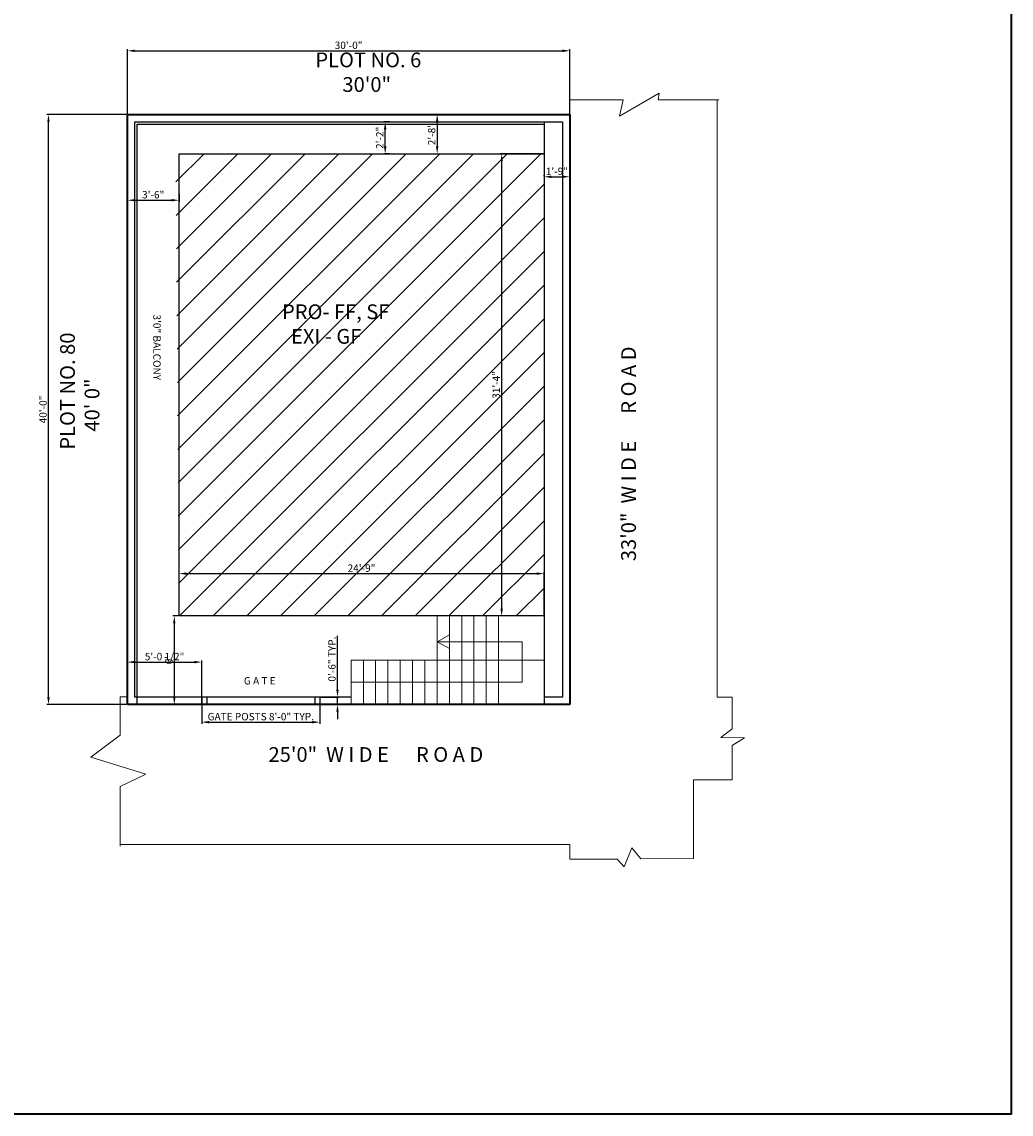
# Model space of a CAD drawing. Units: millimetres. Extents: x 50579 to 52843, y 62224 to 63803.
# Tile 4 of 5: x 52038 to 52843, y 62224 to 63113. Entities that reach past the tile are written whole.
import ezdxf

# ---------------------------------------------------------------- set-up
doc = ezdxf.new("R2010")
doc.units = ezdxf.units.MM
for name, color, linetype, lineweight in [('A-ANNO-DIMS', 2, 'Continuous', 18), ('A-ANNO-TTLB', 7, 'Continuous', 35), ('A-AREA-IDEN', 6, 'Continuous', 18), ('A-FLOR-BALC', 7, 'Continuous', 25), ('A-FLOR-STRS', 7, 'Continuous', 18), ('A-SITE-BLDG', 7, 'Continuous', 25), ('A-SITE-PATT', 8, 'Continuous', 13), ('C-ANNO-TEXT', 4, 'Continuous', 18), ('C-PROP', 7, 'Continuous', 35), ('C-ROAD', 7, 'Continuous', 18), ('C-SITE-GATE', 7, 'Continuous', 25), ('C-SITE-WALL', 7, 'Continuous', 25)]:
    doc.layers.add(name, color=color, linetype=linetype, lineweight=lineweight)
doc.styles.get("Standard").update_dxf_attribs({"font": 'arial.ttf'})
doc.dimstyles.new('ISO-25', dxfattribs={"dimtxt": 6, "dimasz": 6, "dimexe": 1.25, "dimexo": 0.625, "dimtad": 1, "dimdec": 0, "dimlunit": 3, "dimtxsty": 'Standard', "dimcen": 2.5, "dimadec": 0, "dimazin": 0, "dimtfac": 1, "dimtdec": 0, "dimtmove": 0, "dimatfit": 3, "dimfxl": 1, "dimarcsym": 0})

# ---------------------------------------------------------------- blocks, each defined once
blk = doc.blocks.new('*D11')
at = {"layer": 'A-ANNO-DIMS', "color": 0, "lineweight": -2, "transparency": 16777216}
for p, q in [((52123.98, 62972.74), (52123.98, 62966.31)), ((52165.98, 62972.74), (52165.98, 62966.31)), ((52129.98, 62967.56), (52159.98, 62967.56))]:
    blk.add_line(p, q, dxfattribs=at)
at = {"layer": 'A-ANNO-DIMS', "color": 0, "transparency": 16777216}
for points in [[(52129.98, 62968.56), (52129.98, 62966.56), (52123.98, 62967.56)], [(52159.98, 62968.56), (52159.98, 62966.56), (52165.98, 62967.56)]]:
    blk.add_solid(points, dxfattribs=at)
at = {"layer": 'Defpoints', "color": 0, "transparency": 16777216}
for p in [(52123.98, 62973.36), (52165.98, 62973.36), (52165.98, 62967.56)]:
    blk.add_point(p, dxfattribs=at)
at = {"layer": 'A-ANNO-DIMS', "color": 0, "transparency": 16777216, "insert": (52144.98, 62971.25), "char_height": 6, "attachment_point": 5}
blk.add_mtext('3\'-6"', dxfattribs=at)
blk = doc.blocks.new('*D12')
at = {"layer": 'A-ANNO-DIMS', "color": 0, "lineweight": -2, "transparency": 16777216}
for p, q in [((52376.66, 63037.35), (52377.28, 63037.35)), ((52376.03, 63031.35), (52376.03, 63011.35)), ((52376.66, 63005.35), (52377.28, 63005.35))]:
    blk.add_line(p, q, dxfattribs=at)
at = {"layer": 'A-ANNO-DIMS', "color": 0, "transparency": 16777216}
for points in [[(52375.03, 63031.35), (52377.03, 63031.35), (52376.03, 63037.35)], [(52375.03, 63011.35), (52377.03, 63011.35), (52376.03, 63005.35)]]:
    blk.add_solid(points, dxfattribs=at)
at = {"layer": 'Defpoints', "color": 0, "transparency": 16777216}
for p in [(52376.03, 63037.35), (52376.03, 63005.35), (52376.03, 63005.35)]:
    blk.add_point(p, dxfattribs=at)
at = {"layer": 'A-ANNO-DIMS', "color": 0, "transparency": 16777216, "insert": (52372.34, 63021.35), "char_height": 6, "attachment_point": 5, "rotation": 90}
blk.add_mtext('2\'-8"', dxfattribs=at)
blk = doc.blocks.new('*D13')
at = {"layer": 'A-ANNO-DIMS', "color": 0, "lineweight": -2, "transparency": 16777216}
for p, q in [((52337.49, 63031.35), (52332.5, 63031.35)), ((52333.75, 63011.35), (52333.75, 63025.35)), ((52337.49, 63005.35), (52332.5, 63005.35))]:
    blk.add_line(p, q, dxfattribs=at)
at = {"layer": 'A-ANNO-DIMS', "color": 0, "transparency": 16777216}
for points in [[(52332.75, 63025.35), (52334.75, 63025.35), (52333.75, 63031.35)], [(52332.75, 63011.35), (52334.75, 63011.35), (52333.75, 63005.35)]]:
    blk.add_solid(points, dxfattribs=at)
at = {"layer": 'Defpoints', "color": 0, "transparency": 16777216}
for p in [(52333.75, 63031.35), (52338.12, 63031.35), (52338.12, 63005.35)]:
    blk.add_point(p, dxfattribs=at)
at = {"layer": 'A-ANNO-DIMS', "color": 0, "transparency": 16777216, "insert": (52330.12, 63018.35), "char_height": 6, "attachment_point": 5, "rotation": 90}
blk.add_mtext('2\'-2"', dxfattribs=at)
blk = doc.blocks.new('*D14')
at = {"layer": 'A-ANNO-DIMS', "color": 0, "lineweight": -2, "transparency": 16777216}
for p, q in [((52462.98, 62987.28), (52462.98, 62987.91)), ((52468.98, 62986.66), (52477.98, 62986.66)), ((52483.98, 62987.28), (52483.98, 62987.91))]:
    blk.add_line(p, q, dxfattribs=at)
at = {"layer": 'A-ANNO-DIMS', "color": 0, "transparency": 16777216}
for points in [[(52468.98, 62987.66), (52468.98, 62985.66), (52462.98, 62986.66)], [(52477.98, 62987.66), (52477.98, 62985.66), (52483.98, 62986.66)]]:
    blk.add_solid(points, dxfattribs=at)
at = {"layer": 'Defpoints', "color": 0, "transparency": 16777216}
for p in [(52462.98, 62986.66), (52483.98, 62986.66), (52483.98, 62986.66)]:
    blk.add_point(p, dxfattribs=at)
at = {"layer": 'A-ANNO-DIMS', "color": 0, "transparency": 16777216, "insert": (52473.48, 62990.34), "char_height": 6, "attachment_point": 5}
blk.add_mtext('1\'-9"', dxfattribs=at)
blk = doc.blocks.new('*D15')
at = {"layer": 'A-ANNO-DIMS', "color": 0, "lineweight": -2, "transparency": 16777216}
for p, q in [((52165.35, 62629.35), (52160.88, 62629.35)), ((52162.13, 62623.35), (52162.13, 62563.35)), ((52165.35, 62557.35), (52160.88, 62557.35))]:
    blk.add_line(p, q, dxfattribs=at)
at = {"layer": 'A-ANNO-DIMS', "color": 0, "transparency": 16777216}
for points in [[(52161.13, 62623.35), (52163.13, 62623.35), (52162.13, 62629.35)], [(52161.13, 62563.35), (52163.13, 62563.35), (52162.13, 62557.35)]]:
    blk.add_solid(points, dxfattribs=at)
at = {"layer": 'Defpoints', "color": 0, "transparency": 16777216}
for p in [(52165.98, 62629.35), (52162.13, 62557.35), (52165.98, 62557.35)]:
    blk.add_point(p, dxfattribs=at)
at = {"layer": 'A-ANNO-DIMS', "color": 0, "transparency": 16777216, "insert": (52158.44, 62593.35), "char_height": 6, "attachment_point": 5, "rotation": 90}
blk.add_mtext("6'", dxfattribs=at)
blk = doc.blocks.new('GATE-POST-PAIR')
for p, q in [((0, 6), (0, 0)), ((4, 6), (4, 0)), ((92.04, 6), (92.04, 0)), ((96.04, 6), (96.04, 0))]:
    blk.add_line(p, q)
blk = doc.blocks.new('*D35')
at = {"layer": 'A-ANNO-DIMS', "color": 0, "lineweight": -2, "transparency": 16777216}
for p, q in [((52184.48, 62556.73), (52184.48, 62541.7)), ((52280.52, 62556.73), (52280.52, 62541.7)), ((52190.48, 62542.95), (52274.52, 62542.95))]:
    blk.add_line(p, q, dxfattribs=at)
at = {"layer": 'A-ANNO-DIMS', "color": 0, "transparency": 16777216}
for points in [[(52190.48, 62543.95), (52190.48, 62541.95), (52184.48, 62542.95)], [(52274.52, 62543.95), (52274.52, 62541.95), (52280.52, 62542.95)]]:
    blk.add_solid(points, dxfattribs=at)
at = {"layer": 'Defpoints', "color": 0, "transparency": 16777216}
for p in [(52184.48, 62557.35), (52280.52, 62557.35), (52280.52, 62542.95)]:
    blk.add_point(p, dxfattribs=at)
at = {"layer": 'A-ANNO-DIMS', "color": 0, "transparency": 16777216, "insert": (52232.5, 62546.68), "char_height": 6, "attachment_point": 5}
blk.add_mtext('GATE POSTS 8\'-0" TYP.', dxfattribs=at)
blk = doc.blocks.new('*D36')
at = {"layer": 'A-ANNO-DIMS', "color": 0, "lineweight": -2, "transparency": 16777216}
for p, q in [((52294.92, 62569.35), (52294.92, 62613.17)), ((52281.14, 62563.35), (52296.17, 62563.35)), ((52294.92, 62557.35), (52294.92, 62563.35)), ((52281.14, 62557.35), (52296.17, 62557.35)), ((52294.92, 62551.35), (52294.92, 62545.35))]:
    blk.add_line(p, q, dxfattribs=at)
at = {"layer": 'A-ANNO-DIMS', "color": 0, "transparency": 16777216}
for points in [[(52293.92, 62569.35), (52295.92, 62569.35), (52294.92, 62563.35)], [(52293.92, 62551.35), (52295.92, 62551.35), (52294.92, 62557.35)]]:
    blk.add_solid(points, dxfattribs=at)
at = {"layer": 'Defpoints', "color": 0, "transparency": 16777216}
for p in [(52280.52, 62563.35), (52294.92, 62563.35), (52280.52, 62557.35)]:
    blk.add_point(p, dxfattribs=at)
at = {"layer": 'A-ANNO-DIMS', "color": 0, "transparency": 16777216, "insert": (52291.23, 62594.26), "char_height": 6, "attachment_point": 5, "rotation": 90}
blk.add_mtext('0\'-6" TYP.', dxfattribs=at)
blk = doc.blocks.new('*D43')
at = {"layer": 'A-ANNO-DIMS', "color": 0, "lineweight": -2, "transparency": 16777216}
for p, q in [((52123.98, 63037.98), (52123.98, 63090.38)), ((52129.98, 63089.13), (52477.98, 63089.13)), ((52483.98, 63037.98), (52483.98, 63090.38))]:
    blk.add_line(p, q, dxfattribs=at)
at = {"layer": 'A-ANNO-DIMS', "color": 0, "transparency": 16777216}
for points in [[(52129.98, 63090.13), (52129.98, 63088.13), (52123.98, 63089.13)], [(52477.98, 63090.13), (52477.98, 63088.13), (52483.98, 63089.13)]]:
    blk.add_solid(points, dxfattribs=at)
at = {"layer": 'Defpoints', "color": 0, "transparency": 16777216}
for p in [(52483.98, 63089.13), (52123.98, 63037.35), (52483.98, 63037.35)]:
    blk.add_point(p, dxfattribs=at)
at = {"layer": 'A-ANNO-DIMS', "color": 0, "transparency": 16777216, "insert": (52303.98, 63092.82), "char_height": 6, "attachment_point": 5}
blk.add_mtext('30\'-0"', dxfattribs=at)
blk = doc.blocks.new('*D44')
at = {"layer": 'A-ANNO-DIMS', "color": 0, "lineweight": -2, "transparency": 16777216}
for p, q in [((52123.35, 63037.35), (52058.51, 63037.35)), ((52059.76, 62563.35), (52059.76, 63031.35)), ((52123.35, 62557.35), (52058.51, 62557.35))]:
    blk.add_line(p, q, dxfattribs=at)
at = {"layer": 'A-ANNO-DIMS', "color": 0, "transparency": 16777216}
for points in [[(52058.76, 63031.35), (52060.76, 63031.35), (52059.76, 63037.35)], [(52058.76, 62563.35), (52060.76, 62563.35), (52059.76, 62557.35)]]:
    blk.add_solid(points, dxfattribs=at)
at = {"layer": 'Defpoints', "color": 0, "transparency": 16777216}
for p in [(52059.76, 63037.35), (52123.98, 63037.35), (52123.98, 62557.35)]:
    blk.add_point(p, dxfattribs=at)
at = {"layer": 'A-ANNO-DIMS', "color": 0, "transparency": 16777216, "insert": (52056.07, 62797.35), "char_height": 6, "attachment_point": 5, "rotation": 90}
blk.add_mtext('40\'-0"', dxfattribs=at)
blk = doc.blocks.new('*D73')
at = {"layer": 'A-ANNO-DIMS', "color": 0, "lineweight": -2, "transparency": 16777216}
for p, q in [((52123.98, 62557.98), (52123.98, 62593.05)), ((52129.98, 62591.8), (52178.48, 62591.8)), ((52184.48, 62557.98), (52184.48, 62593.05))]:
    blk.add_line(p, q, dxfattribs=at)
at = {"layer": 'A-ANNO-DIMS', "color": 0, "transparency": 16777216}
for points in [[(52129.98, 62592.8), (52129.98, 62590.8), (52123.98, 62591.8)], [(52178.48, 62592.8), (52178.48, 62590.8), (52184.48, 62591.8)]]:
    blk.add_solid(points, dxfattribs=at)
at = {"layer": 'Defpoints', "color": 0, "transparency": 16777216}
for p in [(52184.48, 62591.8), (52123.98, 62557.35), (52184.48, 62557.35)]:
    blk.add_point(p, dxfattribs=at)
at = {"layer": 'A-ANNO-DIMS', "color": 0, "transparency": 16777216, "insert": (52154.23, 62595.53), "char_height": 6, "attachment_point": 5}
blk.add_mtext('5\'-0 1/2"', dxfattribs=at)
blk = doc.blocks.new('*D74')
at = {"layer": 'A-ANNO-DIMS', "color": 0, "lineweight": -2, "transparency": 16777216}
for p, q in [((52165.98, 62629.98), (52165.98, 62665.05)), ((52171.98, 62663.8), (52456.98, 62663.8)), ((52462.98, 62629.98), (52462.98, 62665.05))]:
    blk.add_line(p, q, dxfattribs=at)
at = {"layer": 'A-ANNO-DIMS', "color": 0, "transparency": 16777216}
for points in [[(52171.98, 62664.8), (52171.98, 62662.8), (52165.98, 62663.8)], [(52456.98, 62664.8), (52456.98, 62662.8), (52462.98, 62663.8)]]:
    blk.add_solid(points, dxfattribs=at)
at = {"layer": 'Defpoints', "color": 0, "transparency": 16777216}
for p in [(52462.98, 62663.8), (52165.98, 62629.35), (52462.98, 62629.35)]:
    blk.add_point(p, dxfattribs=at)
at = {"layer": 'A-ANNO-DIMS', "color": 0, "transparency": 16777216, "insert": (52314.48, 62667.49), "char_height": 6, "attachment_point": 5}
blk.add_mtext('24\'-9"', dxfattribs=at)
blk = doc.blocks.new('*D75')
at = {"layer": 'A-ANNO-DIMS', "color": 0, "lineweight": -2, "transparency": 16777216}
for p, q in [((52462.35, 63005.35), (52427.28, 63005.35)), ((52428.53, 62635.35), (52428.53, 62999.35)), ((52462.35, 62629.35), (52427.28, 62629.35))]:
    blk.add_line(p, q, dxfattribs=at)
at = {"layer": 'A-ANNO-DIMS', "color": 0, "transparency": 16777216}
for points in [[(52427.53, 62999.35), (52429.53, 62999.35), (52428.53, 63005.35)], [(52427.53, 62635.35), (52429.53, 62635.35), (52428.53, 62629.35)]]:
    blk.add_solid(points, dxfattribs=at)
at = {"layer": 'Defpoints', "color": 0, "transparency": 16777216}
for p in [(52428.53, 63005.35), (52462.98, 63005.35), (52462.98, 62629.35)]:
    blk.add_point(p, dxfattribs=at)
at = {"layer": 'A-ANNO-DIMS', "color": 0, "transparency": 16777216, "insert": (52424.84, 62817.35), "char_height": 6, "attachment_point": 5, "rotation": 90}
blk.add_mtext('31\'-4"', dxfattribs=at)

msp = doc.modelspace()

# ---------------------------------------------------------------- hatches: boundary and pattern name
at = {"layer": 'A-SITE-PATT'}
h = msp.add_hatch(dxfattribs=at)
h.set_pattern_fill('ANSI31', color=256, scale=6.1)
h.paths.add_polyline_path([(52462.98, 63005.35), (52163.3, 63005.35), (52165.98, 62629.35), (52298.51, 62629.35), (52317.68, 62629.35), (52387.68, 62629.35), (52375.98, 62629.35), (52462.98, 62629.35)])
h.paths.add_polyline_path([(52213.58, 62570.21), (52199.92, 62570.21), (52196.37, 62570.21)])

# ---------------------------------------------------------------- linework, layer by layer
at = {"layer": 'A-ANNO-TTLB'}
msp.add_lwpolyline([(50579.46, 63802.65), (52843.1, 63802.65), (52843.1, 62224.04), (50579.46, 62224.04)], close=True, dxfattribs=at)
at = {"layer": 'A-FLOR-BALC'}
msp.add_line((52462.98, 62629.35), (52462.98, 62557.35), dxfattribs=at)
msp.add_lwpolyline([(52131.98, 62557.35), (52131.98, 63029.35), (52462.98, 63029.35)], dxfattribs=at)
at = {"layer": 'A-FLOR-STRS'}
for p, q in [((52375.98, 62629.35), (52375.98, 62557.35)), ((52385.98, 62629.35), (52385.98, 62557.35)), ((52395.98, 62629.35), (52395.98, 62557.35)), ((52405.98, 62629.35), (52405.98, 62557.35)), ((52415.98, 62629.35), (52415.98, 62557.35)), ((52425.98, 62629.35), (52425.98, 62557.35)), ((52375.98, 62608.36), (52385.98, 62613.89)), ((52445.17, 62608.36), (52375.98, 62608.36)), ((52375.98, 62608.36), (52385.98, 62602.83)), ((52445.17, 62575.35), (52445.17, 62608.36)), ((52305.98, 62593.35), (52462.98, 62593.35)), ((52305.98, 62593.35), (52305.98, 62557.35)), ((52315.98, 62593.35), (52315.98, 62557.35)), ((52325.98, 62593.35), (52325.98, 62557.35)), ((52335.98, 62593.35), (52335.98, 62557.35)), ((52345.98, 62593.35), (52345.98, 62557.35)), ((52355.98, 62593.35), (52355.98, 62557.35)), ((52365.98, 62593.35), (52365.98, 62557.35)), ((52305.98, 62575.35), (52445.17, 62575.35))]:
    msp.add_line(p, q, dxfattribs=at)
at = {"layer": 'A-SITE-BLDG'}
for p, q in [((52462.98, 63031.35), (52462.98, 62629.35)), ((52165.98, 62629.35), (52165.98, 63005.35)), ((52165.98, 63005.35), (52462.98, 63005.35)), ((52462.98, 62629.35), (52165.98, 62629.35))]:
    msp.add_line(p, q, dxfattribs=at)
at = {"layer": 'C-PROP'}
for p, q in [((52123.98, 63037.35), (52483.98, 63037.35)), ((52123.98, 62557.35), (52123.98, 63037.35)), ((52483.98, 63037.35), (52483.98, 62557.35)), ((52483.98, 62557.35), (52123.98, 62557.35))]:
    msp.add_line(p, q, dxfattribs=at)
at = {"layer": 'C-ROAD'}
for p, q in [((52603.98, 63049.35), (52603.98, 62563.35)), ((52603.98, 62563.35), (52615.98, 62563.35)), ((52615.98, 62496.1), (52584.49, 62496.1)), ((52584.49, 62496.1), (52584.49, 62431.93)), ((52483.98, 62443.35), (52117.98, 62443.35)), ((52483.98, 62443.35), (52483.98, 62431.35))]:
    msp.add_line(p, q, dxfattribs=at)
for points in [[(52483.98, 63037.35), (52483.98, 63049.35), (52527.34, 63049.35), (52524.38, 63035.88), (52556.75, 63054.68), (52555.93, 63049.35), (52605.23, 63049.35)], [(52123.98, 62563.58), (52117.98, 62563.58), (52117.98, 62532.29), (52094.21, 62514.45), (52139.06, 62500.69), (52117.98, 62490.48), (52117.98, 62442.1)], [(52615.98, 62563.35), (52615.98, 62537.62), (52606.83, 62530.48), (52626.06, 62530.23), (52615.98, 62523.87), (52615.98, 62496.1)], [(52483.98, 62431.35), (52522.55, 62431.58), (52528.25, 62425.16), (52534.36, 62440.74), (52541.72, 62431.66), (52584.49, 62431.93)]]:
    msp.add_lwpolyline(points, dxfattribs=at)
at = {"layer": 'C-SITE-WALL'}
msp.add_line((52305.98, 62563.35), (52129.98, 62563.35), dxfattribs=at)
msp.add_lwpolyline([(52129.98, 62563.35), (52129.98, 63031.35), (52477.98, 63031.35), (52477.98, 62563.35), (52462.98, 62563.35)], dxfattribs=at)

# ---------------------------------------------------------------- block references
at = {"layer": 'C-SITE-GATE'}
msp.add_blockref('GATE-POST-PAIR', (52184.48, 62557.35), dxfattribs=at)

# ---------------------------------------------------------------- texts
at = {"layer": 'A-AREA-IDEN', "insert": (52151.02, 62878.29), "char_height": 6, "attachment_point": 1, "rotation": 270}
msp.add_mtext_dynamic_manual_height_columns('  3\'0" BALCONY', width=88.9546, gutter_width=12.5, heights=[0], dxfattribs=at)
at = {"layer": 'C-ANNO-TEXT', "attachment_point": 1}
for s, width, insert, char_height in [('  PLOT NO. 6 \\P        30\'0"', 227.2367, (52269.61, 63087.73), 12), ('     PRO- FF, SF\\P       EXI - GF', 227.2367, (52231.47, 62882.84), 12), ('  G A T E', 46.1696, (52215.08, 62579.59), 6), ('  25\'0"  W I D E      R O A D', 227.2367, (52231.47, 62522.64), 12)]:
    msp.add_mtext_dynamic_manual_height_columns(s, width=width, gutter_width=12.5, heights=[0], dxfattribs=dict(at, insert=insert, char_height=char_height))
at = {"layer": 'C-ANNO-TEXT', "char_height": 12, "attachment_point": 1, "rotation": 90}
for s, insert in [('  PLOT NO. 80\\P      40\' 0"', (52069.21, 62757.34)), ('  33\'0"  W I D E      R O A D', (52525.78, 62666.56))]:
    msp.add_mtext_dynamic_manual_height_columns(s, width=227.2367, gutter_width=12.5, heights=[0], dxfattribs=dict(at, insert=insert))

# ---------------------------------------------------------------- dimensions: what is measured, and where the dimension line sits
at = {"layer": 'A-ANNO-DIMS'}
for base, p1, p2, override, picture, middle in [((52483.98, 63089.13), (52123.98, 63037.35), (52483.98, 63037.35), {"dimdec": 1, "dimlfac": 1, "dimrnd": 0, "dimzin": 1, "dimdsep": 46, "dimlunit": 4, "dimfrac": 2}, '*D43', (52303.98, 63092.82)), ((52483.98, 62986.66), (52462.98, 62986.66), (52483.98, 62986.66), {"dimclrd": 0, "dimclre": 0, "dimclrt": 0}, '*D14', (52473.48, 62990.34)), ((52165.98, 62967.56), (52123.98, 62973.36), (52165.98, 62973.36), {"dimclrd": 0, "dimclre": 0, "dimclrt": 0}, '*D11', (52144.98, 62971.25)), ((52184.48, 62591.8), (52123.98, 62557.35), (52184.48, 62557.35), {"dimdec": 1, "dimlfac": 1, "dimrnd": 0, "dimzin": 1, "dimdsep": 46, "dimlunit": 4, "dimfrac": 2}, '*D73', (52154.23, 62595.53))]:
    dim = msp.add_linear_dim(base=base, p1=p1, p2=p2, dimstyle='ISO-25', override=override, dxfattribs=at)
    dim.commit()
    dim.dimension.update_dxf_attribs({"geometry": picture, "text_midpoint": middle})
for base, p1, p2, angle, override, picture, middle in [((52059.76, 63037.35), (52123.98, 62557.35), (52123.98, 63037.35), 90, {"dimdec": 1, "dimlfac": 1, "dimrnd": 0, "dimzin": 1, "dimdsep": 46, "dimlunit": 4, "dimfrac": 2}, '*D44', (52056.07, 62797.35)), ((52376.03, 63005.35), (52376.03, 63037.35), (52376.03, 63005.35), 90, {"dimclrd": 0, "dimclre": 0, "dimclrt": 0}, '*D12', (52372.34, 63021.35)), ((52333.75, 63031.35), (52338.12, 63005.35), (52338.12, 63031.35), 90, {"dimclrd": 0, "dimclre": 0, "dimclrt": 0}, '*D13', (52330.12, 63018.35)), ((52428.53, 63005.35), (52462.98, 62629.35), (52462.98, 63005.35), 90, {"dimdec": 1, "dimlfac": 1, "dimrnd": 0, "dimzin": 1, "dimdsep": 46, "dimlunit": 4, "dimfrac": 2}, '*D75', (52424.84, 62817.35)), ((52462.98, 62663.8), (52165.98, 62629.35), (52462.98, 62629.35), 0, {"dimdec": 1, "dimlfac": 1, "dimrnd": 0, "dimzin": 1, "dimdsep": 46, "dimlunit": 4, "dimfrac": 2}, '*D74', (52314.48, 62667.49)), ((52162.13, 62557.35), (52165.98, 62629.35), (52165.98, 62557.35), 90, {"dimclrd": 0, "dimclre": 0, "dimclrt": 0}, '*D15', (52158.44, 62593.35))]:
    dim = msp.add_linear_dim(base=base, p1=p1, p2=p2, angle=angle, dimstyle='ISO-25', override=override, dxfattribs=at)
    dim.commit()
    dim.dimension.update_dxf_attribs({"geometry": picture, "text_midpoint": middle})
dim = msp.add_linear_dim(base=(52294.92, 62563.35), p1=(52280.52, 62557.35), p2=(52280.52, 62563.35), angle=90, text='<> TYP.', dimstyle='ISO-25', override={"dimdec": 1, "dimlfac": 1, "dimrnd": 0, "dimzin": 1, "dimdsep": 46, "dimlunit": 4, "dimfrac": 2}, dxfattribs=at)
dim.commit()
dim.dimension.update_dxf_attribs({"geometry": '*D36', "text_midpoint": (52291.23, 62594.26)})
dim = msp.add_linear_dim(base=(52280.52, 62542.95), p1=(52184.48, 62557.35), p2=(52280.52, 62557.35), text='GATE POSTS <> TYP.', dimstyle='ISO-25', override={"dimdec": 1, "dimlfac": 1, "dimrnd": 0, "dimzin": 1, "dimdsep": 46, "dimlunit": 4, "dimfrac": 2}, dxfattribs=at)
dim.commit()
dim.dimension.update_dxf_attribs({"geometry": '*D35', "text_midpoint": (52232.5, 62546.68)})

doc.saveas('drawing.dxf')
